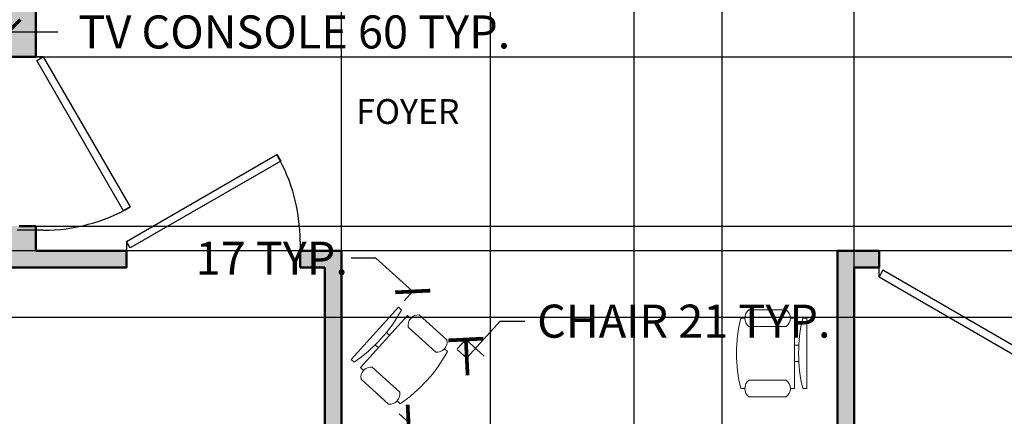
# Model space of a CAD drawing. Units: inches. Extents: x -30 to 744, y -375 to 57.
# Tile 3 of 8: x 116 to 355, y -230 to -134. Entities that reach past the tile are written whole.
import ezdxf

# ---------------------------------------------------------------- set-up
doc = ezdxf.new("R2010")
doc.units = ezdxf.units.IN
doc.header["$MEASUREMENT"] = 0
for name, color, linetype, lineweight in [('A-ANNO-DIMS', 2, 'Continuous', 18), ('A-AREA-IDEN', 7, 'Continuous', 25), ('A-DOOR', 3, 'Continuous', 25), ('A-FURN', 8, 'Continuous', 18), ('A-WALL', 7, 'Continuous', 50)]:
    doc.layers.add(name, color=color, linetype=linetype, lineweight=lineweight)
doc.layers.add('A-WALL-PATT', color=251, linetype='Continuous', lineweight=13, true_color=0x636466)
doc.styles.get("Standard").update_dxf_attribs({"font": 'arial.ttf'})
doc.dimstyles.get("Standard").update_dxf_attribs({"dimtxt": 8, "dimasz": 6, "dimexe": 0.18, "dimexo": 0.0625, "dimgap": 0.09, "dimtad": 0, "dimtih": 1, "dimtoh": 1, "dimdec": 0, "dimzin": 0, "dimdsep": 46, "dimlunit": 4, "dimtxsty": 'Standard', "dimblk": 'ARCHTICK', "dimcen": 0.09, "dimadec": 0, "dimazin": 0, "dimtfac": 1, "dimtdec": 0, "dimtofl": 0, "dimtmove": 0, "dimatfit": 1, "dimldrblk": 'ARCHTICK', "dimfxl": 1, "dimtolj": 1, "dimtzin": 0, "dimarcsym": 0})

# ---------------------------------------------------------------- blocks, each defined once
blk = doc.blocks.new('*U4')
for p, q in [((0, 0), (0, 6)), ((40, 0), (40, 6))]:
    blk.add_line(p, q)
blk.add_lwpolyline([(0, 0), (34.64, -20), (35.52, -18.48), (0.87, 1.52)], close=True)
blk.add_arc((0, 0), 40, 330, 0)
blk = doc.blocks.new('*U2')
for p, q in [((0, 0), (0, -6)), ((40, 0), (40, -6))]:
    blk.add_line(p, q)
blk.add_lwpolyline([(0, 0), (34.64, 20), (35.52, 18.48), (0.87, -1.52)], close=True)
blk.add_arc((0, 0), 40, 0, 30)
blk = doc.blocks.new('Chair - Desk')
for p, q in [((-8.5, 0), (-8.5, -1)), ((-8.5, 0), (8.5, 0)), ((8.5, 0), (8.5, -1)), ((-2, -3), (-2, -1.9355)), ((2, -1.9576), (2, -3)), ((-8.5, -3), (-8.5, -4)), ((-8.5, -3), (8.5, -3)), ((8.5, -3), (8.5, -4)), ((-10.5, -5), (-10.5, -14)), ((-6.5, -14), (-6.5, -5)), ((6.5, -5), (6.5, -14)), ((10.5, -14), (10.5, -5)), ((-8.5, -15), (-8.5, -16)), ((8.5, -15), (8.5, -16))]:
    blk.add_line(p, q)
for centre, radius, start, end in [((0, 34.625), 36.625, 256.5803, 283.4197), ((-8.5, -6.5), 2.5, 36.8699, 143.1301), ((8.5, -6.5), 2.5, 36.8699, 143.1301), ((-8.5, -12.5), 2.5, 216.8699, 323.1301), ((8.5, -12.5), 2.5, 216.8699, 323.1301), ((0, 19.625), 36.625, 256.5803, 283.4197)]:
    blk.add_arc(centre, radius, start, end)
blk = doc.blocks.new('_ArchTick')
at = {"color": 0, "linetype": 'ByBlock', "const_width": 0.15}
blk.add_lwpolyline([(-0.5, -0.5), (0.5, 0.5)], dxfattribs=at)
blk = doc.blocks.new('*D28')
at = {"layer": 'A-ANNO-DIMS', "color": 0, "lineweight": -2, "transparency": 16777216}
for p, q in [((224.53, -216.2), (232.58, -207.3)), ((232.58, -207.3), (238.58, -207.3)), ((222.24, -214.13), (224.66, -216.32)), ((208.15, -229.7), (210.58, -231.89)), ((210.44, -231.77), (206.42, -236.22))]:
    blk.add_line(p, q, dxfattribs=at)
at = {"layer": 'Defpoints', "color": 0, "transparency": 16777216}
for p in [(222.2, -214.08), (224.53, -216.2), (208.11, -229.66)]:
    blk.add_point(p, dxfattribs=at)
at = {"layer": 'A-ANNO-DIMS', "color": 0, "lineweight": -2, "transparency": 16777216, "xscale": 6, "yscale": 6, "zscale": 6}
for p, rotation in [((224.53, -216.2), 227.8616521635315), ((210.44, -231.77), 47.86165216353145)]:
    blk.add_blockref('_ArchTick', p, dxfattribs=dict(at, rotation=rotation))
at = {"layer": 'A-ANNO-DIMS', "color": 0, "transparency": 16777216, "insert": (277.03, -207.3), "char_height": 8, "attachment_point": 5}
blk.add_mtext('\\A1;CHAIR 21 TYP.', dxfattribs=at)
blk = doc.blocks.new('*D29')
at = {"layer": 'A-ANNO-DIMS', "color": 0, "lineweight": -2, "transparency": 16777216}
for p, q in [((202.56, -192.07), (196.56, -192.07)), ((211.46, -200.12), (202.56, -192.07)), ((209.38, -202.41), (211.58, -199.99)), ((222.24, -214.04), (224.43, -211.62)), ((224.31, -211.75), (228.76, -215.77))]:
    blk.add_line(p, q, dxfattribs=at)
at = {"layer": 'Defpoints', "color": 0, "transparency": 16777216}
for p in [(211.46, -200.12), (209.34, -202.46), (222.2, -214.08)]:
    blk.add_point(p, dxfattribs=at)
at = {"layer": 'A-ANNO-DIMS', "color": 0, "lineweight": -2, "transparency": 16777216, "xscale": 6, "yscale": 6, "zscale": 6}
for p, rotation in [((211.46, -200.12), 317.8616521635315), ((224.31, -211.75), 137.8616521635315)]:
    blk.add_blockref('_ArchTick', p, dxfattribs=dict(at, rotation=rotation))
at = {"layer": 'A-ANNO-DIMS', "color": 0, "transparency": 16777216, "insert": (177.37, -192.07), "char_height": 8, "attachment_point": 5}
blk.add_mtext('\\A1;17 TYP.', dxfattribs=at)
blk = doc.blocks.new('*D44')
at = {"layer": 'A-ANNO-DIMS', "color": 0, "lineweight": -2, "transparency": 16777216}
for p, q in [((53.6, -128.37), (53.6, -137.48)), ((113.6, -128.37), (113.6, -137.48)), ((53.6, -137.3), (47.6, -137.3)), ((113.6, -137.3), (125.6, -137.3))]:
    blk.add_line(p, q, dxfattribs=at)
at = {"layer": 'Defpoints', "color": 0, "transparency": 16777216}
for p in [(53.6, -128.3), (113.6, -128.3), (113.6, -137.3)]:
    blk.add_point(p, dxfattribs=at)
at = {"layer": 'A-ANNO-DIMS', "color": 0, "lineweight": -2, "transparency": 16777216, "xscale": 6, "yscale": 6, "zscale": 6}
blk.add_blockref('_ArchTick', (53.6, -137.3), dxfattribs=at)
at = {"layer": 'A-ANNO-DIMS', "color": 0, "lineweight": -2, "transparency": 16777216, "xscale": 6, "yscale": 6, "zscale": 6, "rotation": 180}
blk.add_blockref('_ArchTick', (113.6, -137.3), dxfattribs=at)
at = {"layer": 'A-ANNO-DIMS', "color": 0, "transparency": 16777216, "insert": (182.83, -137.3), "char_height": 8, "attachment_point": 5}
blk.add_mtext('\\A1;TV CONSOLE 60 TYP.', dxfattribs=at)
blk = doc.blocks.new('*D63')
at = {"layer": 'A-ANNO-DIMS', "color": 0, "lineweight": -2, "transparency": 16777216}
for p, q in [((542.17, -132.3), (-16.61, -132.3)), ((-16.43, -132.3), (-16.43, -157.12)), ((-16.43, -190.3), (-16.43, -165.47)), ((542.17, -190.3), (-16.61, -190.3))]:
    blk.add_line(p, q, dxfattribs=at)
at = {"layer": 'Defpoints', "color": 0, "transparency": 16777216}
for p in [(-16.43, -132.3), (542.24, -132.3), (542.24, -190.3)]:
    blk.add_point(p, dxfattribs=at)
at = {"layer": 'A-ANNO-DIMS', "color": 0, "lineweight": -2, "transparency": 16777216, "xscale": 6, "yscale": 6, "zscale": 6}
for p, rotation in [((-16.43, -132.3), 90), ((-16.43, -190.3), 270)]:
    blk.add_blockref('_ArchTick', p, dxfattribs=dict(at, rotation=rotation))
at = {"layer": 'A-ANNO-DIMS', "color": 0, "transparency": 16777216, "insert": (-16.43, -161.3), "char_height": 8, "attachment_point": 5}
blk.add_mtext('\\A1;58', dxfattribs=at)
blk = doc.blocks.new('*D64')
at = {"layer": 'A-ANNO-DIMS', "color": 0, "lineweight": -2, "transparency": 16777216}
for p, q in [((40.3, -206.3), (662.32, -206.3)), ((662.14, -206.3), (662.14, -258.19)), ((662.14, -318.3), (662.14, -266.4)), ((40.3, -318.3), (662.32, -318.3))]:
    blk.add_line(p, q, dxfattribs=at)
at = {"layer": 'Defpoints', "color": 0, "transparency": 16777216}
for p in [(40.24, -206.3), (662.14, -206.3), (40.24, -318.3)]:
    blk.add_point(p, dxfattribs=at)
at = {"layer": 'A-ANNO-DIMS', "color": 0, "lineweight": -2, "transparency": 16777216, "xscale": 6, "yscale": 6, "zscale": 6}
for p, rotation in [((662.14, -206.3), 90), ((662.14, -318.3), 270)]:
    blk.add_blockref('_ArchTick', p, dxfattribs=dict(at, rotation=rotation))
at = {"layer": 'A-ANNO-DIMS', "color": 0, "transparency": 16777216, "insert": (662.14, -262.3), "char_height": 8, "attachment_point": 5}
blk.add_mtext('\\A1;112', dxfattribs=at)
blk = doc.blocks.new('*D73')
at = {"layer": 'A-ANNO-DIMS', "color": 0, "lineweight": -2, "transparency": 16777216}
for p, q in [((194.24, -330.23), (194.24, 51.78)), ((194.24, 51.6), (206.42, 51.6)), ((230.24, 51.6), (218.05, 51.6)), ((230.24, -330.23), (230.24, 51.78))]:
    blk.add_line(p, q, dxfattribs=at)
at = {"layer": 'Defpoints', "color": 0, "transparency": 16777216}
for p in [(230.24, 51.6), (194.24, -330.3), (230.24, -330.3)]:
    blk.add_point(p, dxfattribs=at)
at = {"layer": 'A-ANNO-DIMS', "color": 0, "lineweight": -2, "transparency": 16777216, "xscale": 6, "yscale": 6, "zscale": 6, "rotation": 180}
blk.add_blockref('_ArchTick', (194.24, 51.6), dxfattribs=at)
at = {"layer": 'A-ANNO-DIMS', "color": 0, "lineweight": -2, "transparency": 16777216, "xscale": 6, "yscale": 6, "zscale": 6}
blk.add_blockref('_ArchTick', (230.24, 51.6), dxfattribs=at)
at = {"layer": 'A-ANNO-DIMS', "color": 0, "transparency": 16777216, "insert": (212.24, 51.6), "char_height": 8, "attachment_point": 5}
blk.add_mtext('\\A1;36', dxfattribs=at)
blk = doc.blocks.new('*D74')
at = {"layer": 'A-ANNO-DIMS', "color": 0, "lineweight": -2, "transparency": 16777216}
for p, q in [((318.24, -330.23), (318.24, 51.78)), ((318.24, 51.6), (342.41, 51.6)), ((378.24, 51.6), (354.06, 51.6)), ((378.24, -330.23), (378.24, 51.78))]:
    blk.add_line(p, q, dxfattribs=at)
at = {"layer": 'Defpoints', "color": 0, "transparency": 16777216}
for p in [(378.24, 51.6), (318.24, -330.3), (378.24, -330.3)]:
    blk.add_point(p, dxfattribs=at)
at = {"layer": 'A-ANNO-DIMS', "color": 0, "lineweight": -2, "transparency": 16777216, "xscale": 6, "yscale": 6, "zscale": 6, "rotation": 180}
blk.add_blockref('_ArchTick', (318.24, 51.6), dxfattribs=at)
at = {"layer": 'A-ANNO-DIMS', "color": 0, "lineweight": -2, "transparency": 16777216, "xscale": 6, "yscale": 6, "zscale": 6}
blk.add_blockref('_ArchTick', (378.24, 51.6), dxfattribs=at)
at = {"layer": 'A-ANNO-DIMS', "color": 0, "transparency": 16777216, "insert": (348.24, 51.6), "char_height": 8, "attachment_point": 5}
blk.add_mtext('\\A1;60', dxfattribs=at)
blk = doc.blocks.new('*D80')
at = {"layer": 'A-ANNO-DIMS', "color": 0, "lineweight": -2, "transparency": 16777216}
for p, q in [((120.38, -143.3), (662.32, -143.3)), ((662.14, -143.3), (662.14, -159.69)), ((662.14, -184.3), (662.14, -167.9)), ((120.38, -184.3), (662.32, -184.3))]:
    blk.add_line(p, q, dxfattribs=at)
at = {"layer": 'Defpoints', "color": 0, "transparency": 16777216}
for p in [(120.31, -143.3), (662.14, -143.3), (120.31, -184.3)]:
    blk.add_point(p, dxfattribs=at)
at = {"layer": 'A-ANNO-DIMS', "color": 0, "lineweight": -2, "transparency": 16777216, "xscale": 6, "yscale": 6, "zscale": 6}
for p, rotation in [((662.14, -143.3), 90), ((662.14, -184.3), 270)]:
    blk.add_blockref('_ArchTick', p, dxfattribs=dict(at, rotation=rotation))
at = {"layer": 'A-ANNO-DIMS', "color": 0, "transparency": 16777216, "insert": (662.14, -163.8), "char_height": 8, "attachment_point": 5}
blk.add_mtext('\\A1;41', dxfattribs=at)
blk = doc.blocks.new('*D89')
at = {"layer": 'A-ANNO-DIMS', "color": 0, "lineweight": -2, "transparency": 16777216}
for p, q in [((264.9, -64.36), (264.9, -370.38)), ((286.24, -64.36), (286.24, -370.38)), ((264.9, -370.2), (258.9, -370.2)), ((286.24, -370.2), (298.24, -370.2))]:
    blk.add_line(p, q, dxfattribs=at)
at = {"layer": 'Defpoints', "color": 0, "transparency": 16777216}
for p in [(264.9, -64.3), (286.24, -64.3), (286.24, -370.2)]:
    blk.add_point(p, dxfattribs=at)
at = {"layer": 'A-ANNO-DIMS', "color": 0, "lineweight": -2, "transparency": 16777216, "xscale": 6, "yscale": 6, "zscale": 6}
blk.add_blockref('_ArchTick', (264.9, -370.2), dxfattribs=at)
at = {"layer": 'A-ANNO-DIMS', "color": 0, "lineweight": -2, "transparency": 16777216, "xscale": 6, "yscale": 6, "zscale": 6, "rotation": 180}
blk.add_blockref('_ArchTick', (286.24, -370.2), dxfattribs=at)
at = {"layer": 'A-ANNO-DIMS', "color": 0, "transparency": 16777216, "insert": (311.88, -370.2), "char_height": 8, "attachment_point": 5}
blk.add_mtext('\\A1;21.34', dxfattribs=at)

msp = doc.modelspace()

# ---------------------------------------------------------------- hatches: boundary and pattern name
at = {"layer": 'A-WALL-PATT'}
h = msp.add_hatch(color=256, dxfattribs=at)
h.dxf.hatch_style = 1
h.paths.add_polyline_path([(40.2356, 11.7031), (204.2356, 11.7031), (204.2356, -24.2969), (208.2356, -24.2969), (208.2356, 11.7031), (233.4275, 11.7031), (233.4275, 20.7031), (31.2356, 20.7031), (31.2356, -34.2969), (40.2356, -34.2969)])
h.paths.add_polyline_path([(40.2356, -82.2969), (31.2356, -82.2969), (31.2356, -132.2969), (40.2356, -132.2969), (51.0767, -132.2969), (111.3137, -132.2969), (111.3137, -143.2969), (120.3137, -143.2969), (120.3137, -132.2969), (156.2356, -132.2969), (156.2356, -128.2969), (113.6001, -128.2969), (113.6001, -128.3034), (53.6001, -128.3034), (40.2356, -128.2969)])
h.paths.add_polyline_path([(302.4681, 20.7031), (257.4275, 20.7031), (257.4275, 11.7031), (286.2356, 11.7031), (286.2356, -60.2969), (208.2356, -60.2969), (208.2356, -54.2969), (204.2356, -54.2969), (204.2356, -64.2969), (208.2356, -64.2969), (286.2356, -64.2969), (286.2356, -128.2969), (264.8954, -128.2969), (208.2356, -128.2969), (204.2356, -128.2969), (198.2356, -128.2969), (198.2356, -132.2969), (290.2356, -132.2969), (290.2356, -128.2969), (290.2356, 11.7031), (302.4681, 11.7031)])
h.paths.add_polyline_path([(405.515, 20.7031), (350.4681, 20.7031), (350.4681, 11.7031), (362.2356, 11.7031), (362.2356, -34.2969), (366.2356, -34.2969), (366.2356, 11.7031), (405.515, 11.7031)])
h.paths.add_polyline_path([(530.2713, 20.7031), (453.515, 20.7031), (453.515, 11.7031), (486.2356, 11.7031), (486.2356, -128.2969), (448.2356, -128.2969), (448.2356, -132.2969), (486.2356, -132.2969), (490.2356, -132.2969), (496.2356, -132.2969), (496.2356, -128.2969), (490.2356, -128.2969), (490.2356, 11.7031), (530.2713, 11.7031)])
h.paths.add_polyline_path([(631.2356, 20.7031), (578.2713, 20.7031), (578.2713, 11.7031), (622.2356, 11.7031), (622.2356, -37.4001), (631.2356, -37.4001)])
h.paths.add_polyline_path([(631.2356, -85.4001), (622.2356, -85.4001), (622.2356, -91.4001), (622.2356, -103.4001), (622.2356, -128.2969), (538.2356, -128.2969), (538.2356, -132.2969), (538.2356, -154.2969), (542.2356, -154.2969), (542.2356, -132.2969), (575.1375, -132.2969), (585.6313, -131.9348), (585.6438, -132.2969), (622.2356, -132.2969), (622.2356, -147.2969), (631.2356, -147.2969)])
h.paths.add_polyline_path([(631.2356, -171.2969), (622.2356, -171.2969), (622.2356, -185.4028), (622.2356, -186.2969), (622.2356, -190.2969), (542.2356, -190.2969), (542.2356, -184.2969), (538.2356, -184.2969), (538.2356, -190.2969), (538.2356, -194.2969), (622.2356, -194.2969), (622.2356, -237.4632), (631.2356, -237.4632)])
h.paths.add_polyline_path([(631.2356, -285.4632), (622.2356, -285.4632), (622.2356, -330.2969), (490.2356, -330.2969), (490.2356, -194.2969), (494.2356, -194.2969), (495.2356, -194.2969), (495.2356, -190.2969), (494.2356, -190.2969), (490.2356, -190.2969), (486.2356, -190.2969), (366.2356, -190.2969), (366.2356, -194.2969), (486.2356, -194.2969), (486.2356, -330.2969), (426.2356, -330.2969), (426.2356, -339.2969), (631.2356, -339.2969)])
h.paths.add_polyline_path([(378.2356, -330.2969), (318.2356, -330.2969), (318.2356, -194.2969), (324.2356, -194.2969), (324.2356, -190.2969), (318.2356, -190.2969), (314.2356, -190.2969), (314.2356, -194.2969), (314.2356, -330.2969), (278.2356, -330.2969), (278.2356, -339.2969), (378.2356, -339.2969)])
h.paths.add_polyline_path([(190.2356, -330.2969), (40.2356, -330.2969), (40.2356, -318.2969), (31.2356, -318.2969), (31.2356, -330.2969), (31.2356, -339.2969), (190.2356, -339.2969)])
h.paths.add_polyline_path([(230.2356, -330.2969), (194.2356, -330.2969), (194.2356, -194.2969), (194.2356, -190.2969), (190.2356, -190.2969), (184.2356, -190.2969), (184.2356, -194.2969), (190.2356, -194.2969), (190.2356, -339.2969), (230.2356, -339.2969)])
h.paths.add_polyline_path([(142.2356, -190.2969), (120.3137, -190.2969), (120.3137, -184.2969), (116.3137, -184.2969), (111.3137, -184.2969), (111.3137, -190.2969), (40.2356, -190.2969), (31.2356, -190.2969), (31.2356, -194.2969), (31.2356, -206.2969), (40.2356, -206.2969), (40.2356, -194.2969), (142.2356, -194.2969)])

# ---------------------------------------------------------------- linework, layer by layer
at = {"layer": 'A-WALL'}
for p, q in [((120.3137, -143.2969), (120.3137, -132.2969)), ((120.3137, -143.2969), (111.3137, -143.2969)), ((120.3137, -184.2969), (116.3137, -184.2969)), ((120.3137, -190.2969), (120.3137, -184.2969)), ((142.2356, -190.2969), (120.3137, -190.2969)), ((142.2356, -194.2969), (142.2356, -190.2969)), ((190.2356, -190.2969), (184.2356, -190.2969)), ((184.2356, -194.2969), (184.2356, -190.2969)), ((190.2356, -190.2969), (194.2356, -190.2969)), ((194.2356, -190.2969), (194.2356, -194.2969)), ((318.2356, -190.2969), (314.2356, -190.2969)), ((314.2356, -190.2969), (314.2356, -194.2969)), ((318.2356, -190.2969), (324.2356, -190.2969)), ((324.2356, -190.2969), (324.2356, -194.2969)), ((142.2356, -194.2969), (40.2356, -194.2969)), ((190.2356, -194.2969), (184.2356, -194.2969)), ((190.2356, -194.2969), (190.2356, -330.2969)), ((194.2356, -194.2969), (194.2356, -330.2969)), ((314.2356, -194.2969), (314.2356, -330.2969)), ((318.2356, -194.2969), (318.2356, -330.2969)), ((318.2356, -194.2969), (324.2356, -194.2969))]:
    msp.add_line(p, q, dxfattribs=at)

# ---------------------------------------------------------------- block references
at = {"layer": 'A-DOOR', "xscale": 1.05, "yscale": 1.05, "zscale": 1.05, "rotation": 270}
msp.add_blockref('*U2', (122.1137, -143.2969), dxfattribs=at)
at = {"layer": 'A-DOOR', "xscale": 1.05, "yscale": 1.05, "zscale": 1.05}
for name, p in [('*U2', (142.2356, -187.9969)), ('*U4', (324.2356, -196.5969))]:
    msp.add_blockref(name, p, dxfattribs=at)
at = {"layer": 'A-FURN'}
for p, rotation in [((202.2973, -210.2411), 47.86165216353146), ((306.7926, -215.0926), 270)]:
    msp.add_blockref('Chair - Desk', p, dxfattribs=dict(at, rotation=rotation))

# ---------------------------------------------------------------- texts
at = {"layer": 'A-AREA-IDEN', "insert": (197.7962, -153.5573), "char_height": 6, "attachment_point": 1}
msp.add_mtext_dynamic_manual_height_columns('FOYER', width=205.468382, gutter_width=1, heights=[0], dxfattribs=at)

# ---------------------------------------------------------------- dimensions: what is measured, and where the dimension line sits
at = {"layer": 'A-ANNO-DIMS'}
for base, p1, p2, override, picture, middle in [((230.2356, 51.6031), (194.2356, -330.2969), (230.2356, -330.2969), {"dimdec": 0, "dimlfac": 1, "dimrnd": 0, "dimzin": 0, "dimdsep": 46, "dimlunit": 2}, '*D73', (212.2356, 51.6031)), ((378.2356, 51.6031), (318.2356, -330.2969), (378.2356, -330.2969), {"dimdec": 0, "dimlfac": 1, "dimrnd": 0, "dimzin": 0, "dimdsep": 46, "dimlunit": 2}, '*D74', (348.2356, 51.6031)), ((286.2356, -370.1969), (264.8954, -64.2969), (286.2356, -64.2969), {"dimdec": 2, "dimlfac": 1, "dimrnd": 0, "dimzin": 0, "dimdsep": 46, "dimlunit": 2}, '*D89', (311.8754, -370.1969))]:
    dim = msp.add_linear_dim(base=base, p1=p1, p2=p2, dimstyle='Standard', override=override, dxfattribs=at)
    dim.commit()
    dim.dimension.update_dxf_attribs({"geometry": picture, "text_midpoint": middle})
dim = msp.add_linear_dim(base=(113.6001, -137.3034), p1=(53.6001, -128.3034), p2=(113.6001, -128.3034), text='TV CONSOLE <> TYP.', dimstyle='Standard', override={"dimdec": 0, "dimlfac": 1, "dimrnd": 0, "dimzin": 0, "dimdsep": 46, "dimlunit": 2}, dxfattribs=at)
dim.commit()
dim.dimension.update_dxf_attribs({"geometry": '*D44', "text_midpoint": (182.8334, -137.3034)})
for base, p1, p2, picture, middle in [((-16.4253, -132.2969), (542.2356, -190.2969), (542.2356, -132.2969), '*D63', (-16.4253, -161.2969)), ((662.1356, -143.2969), (120.3137, -184.2969), (120.3137, -143.2969), '*D80', (662.1356, -163.7969)), ((662.1356, -206.2969), (40.2356, -318.2969), (40.2356, -206.2969), '*D64', (662.1356, -262.2969))]:
    dim = msp.add_linear_dim(base=base, p1=p1, p2=p2, angle=90, dimstyle='Standard', override={"dimdec": 0, "dimlfac": 1, "dimrnd": 0, "dimzin": 0, "dimdsep": 46, "dimlunit": 2}, dxfattribs=at)
    dim.commit()
    dim.dimension.update_dxf_attribs({"geometry": picture, "text_midpoint": middle})
for base, p1, p2, angle, text, picture, middle in [((211.4554, -200.1193), (222.1951, -214.0844), (209.342, -202.4551), 137.861652, '<> TYP.', '*D29', (177.3729, -192.0682)), ((224.5309, -216.1978), (208.1057, -229.6565), (222.1951, -214.0844), 47.861652, 'CHAIR <> TYP.', '*D28', (277.0349, -207.2995))]:
    dim = msp.add_linear_dim(base=base, p1=p1, p2=p2, angle=angle, text=text, dimstyle='Standard', override={"dimdec": 0, "dimlfac": 1, "dimrnd": 0, "dimzin": 0, "dimdsep": 46, "dimlunit": 2}, dxfattribs=at)
    dim.commit()
    dim.dimension.update_dxf_attribs({"geometry": picture, "text_midpoint": middle})

doc.saveas('drawing.dxf')
